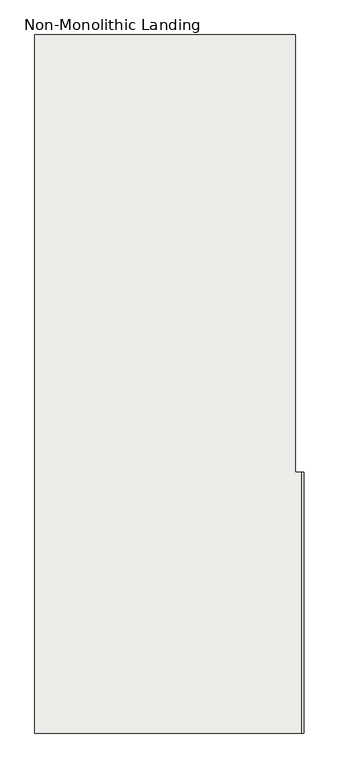
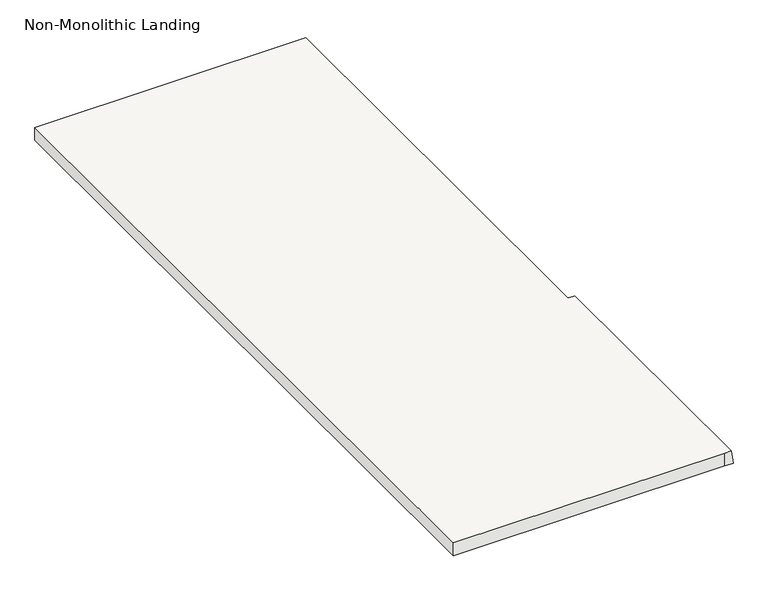
"""IFC4 building model written with IfcOpenShell, lengths in millimetres: slab geometry, Non-Monolithic Landing."""

from ifc_helpers import new_model, si_unit, origin, place, context, project, spatial, faceted_brep, source, transform, mapped, element, save


def non_monolithic_landing_c0ded7b7(model_context):
    return source(origin(), model_context, "Body", "Brep", [
        faceted_brep([(-10449.8492596, 3570.530447, 1565.2173913), (-10442.6617596, 3570.530447, 1515.2173913), (-10442.6617596, 4570.5562283, 1515.2173913), (-10449.8492596, 4570.5562283, 1565.2173913), (-10474.8492596, 6246.9562283, 1565.2173913), (-11474.8750408, 6246.9562283, 1565.2173913), (-11474.8750408, 3570.530447, 1565.2173913), (-10474.8492596, 3570.530447, 1565.2173913), (-10474.8492596, 4570.5562283, 1565.2173913), (-10474.8492596, 5246.930447, 1565.2173913), (-11474.8750408, 3570.530447, 1515.2173913), (-11474.8750408, 6246.9562283, 1515.2173913), (-10482.0367596, 6246.9562283, 1515.2173913), (-10482.0367596, 5246.930447, 1515.2173913), (-10474.8492596, 5246.930447, 1515.2173913), (-10474.8492596, 4570.5562283, 1515.2173913), (-10474.8492596, 3570.530447, 1515.2173913)], [[[0, 1, 2, 3]], [[4, 5, 6, 7, 0, 3, 8, 9]], [[10, 11, 12, 13, 14, 15, 2, 1, 16]], [[5, 4, 12, 11]], [[6, 5, 11, 10]], [[7, 6, 10, 16]], [[0, 7, 16, 1]], [[8, 3, 2, 15]], [[9, 8, 15, 14]], [[13, 9, 14]], [[9, 13, 12, 4]]]),
    ])


if __name__ == "__main__":
    model = new_model("IFC4")
    model_context = context("Model", 3, world=origin())
    ifc_project = project(units=[si_unit("LENGTHUNIT", "METRE", prefix="MILLI")], contexts=[model_context])
    site = spatial("IfcSite", under=ifc_project)
    building = spatial("IfcBuilding", under=site)
    placement = place(None, origin())
    non_monolithic_landing_shape = non_monolithic_landing_c0ded7b7(model_context)
    element("IfcSlab", 1, ObjectType="Non-Monolithic Landing", at=placement, inside=building, context=model_context, shape_type="MappedRepresentation", body=[
        mapped(non_monolithic_landing_shape, transform((0.0, 0.0, 0.0), x_axis=(1.0, 0.0, 0.0), y_axis=(0.0, 1.0, 0.0), z_axis=(0.0, 0.0, 1.0))),
    ])
    save(model, "model.ifc")
